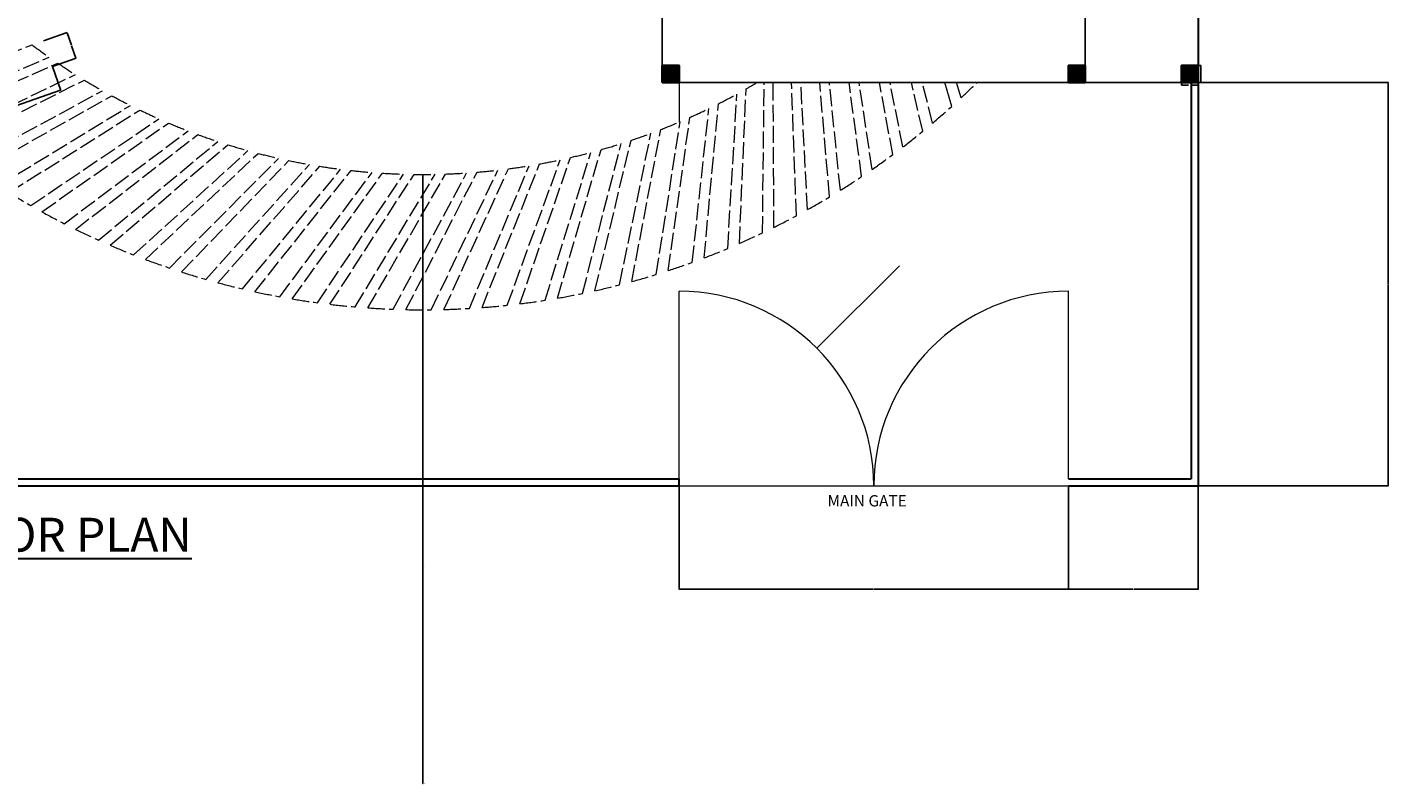
# Model space of a CAD drawing. Units: inches. Extents: x 2330 to 3943, y 1763 to 3461.
# Tile 12 of 40: x 2977 to 3943, y 1763 to 2300. Entities that reach past the tile are written whole.
import ezdxf

# ---------------------------------------------------------------- set-up
doc = ezdxf.new("R2010")
doc.units = ezdxf.units.IN
doc.linetypes.add('ACAD_ISO02W100', pattern=[15, 12, -3])
for name, color, linetype, lineweight in [('A-ANNO-DIMS', 2, 'Continuous', 18), ('A-ANNO-TEXT', 7, 'Continuous', 18), ('A-ANNO-TITL', 7, 'Continuous', 30), ('A-COLS', 7, 'Continuous', 35), ('A-FLOR', 7, 'Continuous', 25), ('C-PROP', 7, 'Continuous', 30), ('L-GATE', 4, 'Continuous', 18), ('L-PVMT', 9, 'Continuous', 18), ('L-PVMT-JOIN', 9, 'ACAD_ISO02W100', 13)]:
    doc.layers.add(name, color=color, linetype=linetype, lineweight=lineweight)
doc.styles.get("Standard").update_dxf_attribs({"font": 'arial.ttf'})
doc.dimstyles.get("Standard").update_dxf_attribs({"dimtxt": 0.18, "dimasz": 0.18, "dimexe": 0.18, "dimexo": 0.0625, "dimgap": 0.09, "dimtad": 0, "dimtih": 1, "dimtoh": 1, "dimdec": 4, "dimzin": 0, "dimdsep": 46, "dimtxsty": 'Standard', "dimcen": 0.09, "dimadec": 0, "dimazin": 0, "dimtfac": 1, "dimtdec": 4, "dimtofl": 0, "dimtmove": 0, "dimatfit": 3, "dimfxl": 1, "dimtolj": 1, "dimtzin": 0, "dimarcsym": 0})

# ---------------------------------------------------------------- blocks, each defined once
blk = doc.blocks.new('PAVER-RADIAL')
for p, q in [((0, 15.76), (109.7, 19.29)), ((8.7, 0), (118.23, 7.05))]:
    blk.add_line(p, q)
for radius, start, end in [(559.83, 207.9852, 209.8274), (463.83, 213.96986, 215.81207)]:
    blk.add_arc((494.37, 278.45), radius, start, end)
blk = doc.blocks.new('POST-PORCH-12IN')
h = blk.add_hatch(color=256)
h.dxf.hatch_style = 1
h.paths.add_polyline_path([(12, 12), (0, 12), (0, 0), (12, 0)])
blk.add_lwpolyline([(0, 0), (12, 0), (12, 12), (0, 12)], close=True)
blk = doc.blocks.new('*D25')
at = {"layer": 'A-ANNO-DIMS', "color": 0, "lineweight": -2, "transparency": 16777216}
for p, q in [((2994.99, 2271.94), (3000.9, 2255.1)), ((3000.67, 2255.21), (2945.58, 2235.87)), ((2883.43, 2232.78), (2889.34, 2215.93)), ((2889.45, 2216.16), (2944.54, 2235.5))]:
    blk.add_line(p, q, dxfattribs=at)
at = {"layer": 'A-ANNO-DIMS', "color": 0, "transparency": 16777216}
for points in [[(3000.66, 2255.23), (3000.68, 2255.18), (3000.84, 2255.27)], [(2889.44, 2216.19), (2889.46, 2216.14), (2889.28, 2216.1)]]:
    blk.add_solid(points, dxfattribs=at)
at = {"layer": 'Defpoints', "color": 0, "transparency": 16777216}
for p in [(2994.96, 2272), (3000.84, 2255.27), (2883.41, 2232.84)]:
    blk.add_point(p, dxfattribs=at)
at = {"layer": 'A-ANNO-DIMS', "color": 0, "transparency": 16777216, "insert": (2945.06, 2235.69), "char_height": 0.18, "attachment_point": 5}
blk.add_mtext('\\A1;PAVER 118 TYP.', dxfattribs=at)
blk = doc.blocks.new('*D26')
at = {"layer": 'A-ANNO-DIMS', "color": 0, "lineweight": -2, "transparency": 16777216}
for p, q in [((2988.64, 2290.22), (3005.48, 2296.13)), ((3005.37, 2295.9), (3008.44, 2287.15)), ((3011.64, 2278.04), (3008.57, 2286.79)), ((2995.02, 2272.02), (3011.87, 2277.93))]:
    blk.add_line(p, q, dxfattribs=at)
at = {"layer": 'A-ANNO-DIMS', "color": 0, "transparency": 16777216}
for points in [[(3005.4, 2295.91), (3005.34, 2295.89), (3005.31, 2296.07)], [(3011.67, 2278.05), (3011.61, 2278.03), (3011.7, 2277.87)]]:
    blk.add_solid(points, dxfattribs=at)
at = {"layer": 'Defpoints', "color": 0, "transparency": 16777216}
for p in [(2988.58, 2290.2), (3005.31, 2296.07), (2994.96, 2272)]:
    blk.add_point(p, dxfattribs=at)
at = {"layer": 'A-ANNO-DIMS', "color": 0, "transparency": 16777216, "insert": (3008.5, 2286.97), "char_height": 0.18, "attachment_point": 5}
blk.add_mtext('\\A1;19 TYP.', dxfattribs=at)
blk = doc.blocks.new('*D29')
at = {"layer": 'A-ANNO-DIMS', "color": 0, "lineweight": -2, "transparency": 16777216}
for p, q in [((3795.66, 2260.64), (3795.66, 2258.72)), ((3807.66, 2260.64), (3807.66, 2258.72)), ((3795.84, 2258.9), (3800.76, 2258.9)), ((3807.48, 2258.9), (3802.56, 2258.9))]:
    blk.add_line(p, q, dxfattribs=at)
at = {"layer": 'A-ANNO-DIMS', "color": 0, "transparency": 16777216}
for points in [[(3795.84, 2258.93), (3795.84, 2258.87), (3795.66, 2258.9)], [(3807.48, 2258.93), (3807.48, 2258.87), (3807.66, 2258.9)]]:
    blk.add_solid(points, dxfattribs=at)
at = {"layer": 'Defpoints', "color": 0, "transparency": 16777216}
for p in [(3795.66, 2260.7), (3807.66, 2260.7), (3807.66, 2258.9)]:
    blk.add_point(p, dxfattribs=at)
at = {"layer": 'A-ANNO-DIMS', "color": 0, "transparency": 16777216, "insert": (3801.66, 2258.9), "char_height": 0.18, "attachment_point": 5}
blk.add_mtext('\\A1;POST 12 TYP.', dxfattribs=at)
blk = doc.blocks.new('*D30')
at = {"layer": 'A-ANNO-DIMS', "color": 0, "lineweight": -2, "transparency": 16777216}
for p, q in [((3807.72, 2272.7), (3809.64, 2272.7)), ((3809.46, 2272.52), (3809.46, 2266.88)), ((3807.72, 2260.7), (3809.64, 2260.7)), ((3809.46, 2260.88), (3809.46, 2266.52))]:
    blk.add_line(p, q, dxfattribs=at)
at = {"layer": 'A-ANNO-DIMS', "color": 0, "transparency": 16777216}
for points in [[(3809.43, 2272.52), (3809.49, 2272.52), (3809.46, 2272.7)], [(3809.43, 2260.88), (3809.49, 2260.88), (3809.46, 2260.7)]]:
    blk.add_solid(points, dxfattribs=at)
at = {"layer": 'Defpoints', "color": 0, "transparency": 16777216}
for p in [(3807.66, 2272.7), (3809.46, 2272.7), (3807.66, 2260.7)]:
    blk.add_point(p, dxfattribs=at)
at = {"layer": 'A-ANNO-DIMS', "color": 0, "transparency": 16777216, "insert": (3809.46, 2266.7), "char_height": 0.18, "attachment_point": 5}
blk.add_mtext('\\A1;12 TYP.', dxfattribs=at)
blk = doc.blocks.new('*D65')
at = {"layer": 'A-ANNO-DIMS', "color": 0, "lineweight": -2, "transparency": 16777216}
for p, q in [((3439.52, 1974.59), (3439.52, 1901.2)), ((3715.52, 1974.59), (3715.52, 1901.2)), ((3439.7, 1901.38), (3577.23, 1901.38)), ((3715.34, 1901.38), (3577.81, 1901.38))]:
    blk.add_line(p, q, dxfattribs=at)
at = {"layer": 'A-ANNO-DIMS', "color": 0, "transparency": 16777216}
for points in [[(3439.7, 1901.41), (3439.7, 1901.35), (3439.52, 1901.38)], [(3715.34, 1901.41), (3715.34, 1901.35), (3715.52, 1901.38)]]:
    blk.add_solid(points, dxfattribs=at)
at = {"layer": 'Defpoints', "color": 0, "transparency": 16777216}
for p in [(3439.52, 1974.65), (3715.52, 1974.65), (3715.52, 1901.38)]:
    blk.add_point(p, dxfattribs=at)
at = {"layer": 'A-ANNO-DIMS', "color": 0, "transparency": 16777216, "insert": (3577.52, 1901.38), "char_height": 0.18, "attachment_point": 5}
blk.add_mtext('\\A1;276', dxfattribs=at)
blk = doc.blocks.new('*D66')
at = {"layer": 'A-ANNO-DIMS', "color": 0, "lineweight": -2, "transparency": 16777216}
for p, q in [((3715.52, 1974.59), (3715.52, 1901.2)), ((3807.66, 1974.59), (3807.66, 1901.2)), ((3715.7, 1901.38), (3761.19, 1901.38)), ((3807.48, 1901.38), (3761.98, 1901.38))]:
    blk.add_line(p, q, dxfattribs=at)
at = {"layer": 'A-ANNO-DIMS', "color": 0, "transparency": 16777216}
for points in [[(3715.7, 1901.41), (3715.7, 1901.35), (3715.52, 1901.38)], [(3807.48, 1901.41), (3807.48, 1901.35), (3807.66, 1901.38)]]:
    blk.add_solid(points, dxfattribs=at)
at = {"layer": 'Defpoints', "color": 0, "transparency": 16777216}
for p in [(3715.52, 1974.65), (3807.66, 1974.65), (3807.66, 1901.38)]:
    blk.add_point(p, dxfattribs=at)
at = {"layer": 'A-ANNO-DIMS', "color": 0, "transparency": 16777216, "insert": (3761.59, 1901.38), "char_height": 0.18, "attachment_point": 5}
blk.add_mtext('\\A1;92.14', dxfattribs=at)
blk = doc.blocks.new('*D68')
at = {"layer": 'A-ANNO-DIMS', "color": 0, "lineweight": -2, "transparency": 16777216}
for p, q in [((3807.72, 2260.7), (3942.54, 2260.7)), ((3942.36, 2260.52), (3942.36, 2117.86)), ((3942.36, 1974.83), (3942.36, 2117.5)), ((3807.72, 1974.65), (3942.54, 1974.65))]:
    blk.add_line(p, q, dxfattribs=at)
at = {"layer": 'A-ANNO-DIMS', "color": 0, "transparency": 16777216}
for points in [[(3942.33, 2260.52), (3942.39, 2260.52), (3942.36, 2260.7)], [(3942.33, 1974.83), (3942.39, 1974.83), (3942.36, 1974.65)]]:
    blk.add_solid(points, dxfattribs=at)
at = {"layer": 'Defpoints', "color": 0, "transparency": 16777216}
for p in [(3807.66, 2260.7), (3942.36, 2260.7), (3807.66, 1974.65)]:
    blk.add_point(p, dxfattribs=at)
at = {"layer": 'A-ANNO-DIMS', "color": 0, "transparency": 16777216, "insert": (3942.36, 2117.68), "char_height": 0.18, "attachment_point": 5}
blk.add_mtext('\\A1;286.05', dxfattribs=at)
blk = doc.blocks.new('*D103')
at = {"layer": 'A-ANNO-DIMS', "color": 0, "lineweight": -2, "transparency": 16777216}
for p, q in [((3257.55, 2659.32), (3257.73, 2659.32)), ((3257.64, 2659.23), (3257.64, 2659.41)), ((3257.66, 1763.59), (3257.65, 2099.31)), ((3257.84, 1763.59), (3257.66, 1763.59))]:
    blk.add_line(p, q, dxfattribs=at)
at = {"layer": 'A-ANNO-DIMS', "color": 0, "transparency": 16777216}
blk.add_solid([(3257.68, 2099.31), (3257.62, 2099.31), (3257.65, 2099.49)], dxfattribs=at)
at = {"layer": 'Defpoints', "color": 0, "transparency": 16777216}
for p in [(3257.64, 2659.32), (3257.65, 2099.49)]:
    blk.add_point(p, dxfattribs=at)
at = {"layer": 'A-ANNO-DIMS', "color": 0, "transparency": 16777216, "insert": (3258.58, 1763.59), "char_height": 0.18, "attachment_point": 5}
blk.add_mtext('\\A1;40X R559.8', dxfattribs=at)
blk = doc.blocks.new('*D104')
at = {"layer": 'A-ANNO-DIMS', "color": 0, "lineweight": -2, "transparency": 16777216}
for p, q in [((3257.55, 2659.32), (3257.73, 2659.32)), ((3257.64, 2659.23), (3257.64, 2659.41)), ((3257.66, 1917.19), (3257.65, 2195.31)), ((3257.84, 1917.19), (3257.66, 1917.19))]:
    blk.add_line(p, q, dxfattribs=at)
at = {"layer": 'A-ANNO-DIMS', "color": 0, "transparency": 16777216}
blk.add_solid([(3257.68, 2195.31), (3257.62, 2195.31), (3257.65, 2195.49)], dxfattribs=at)
at = {"layer": 'Defpoints', "color": 0, "transparency": 16777216}
for p in [(3257.64, 2659.32), (3257.65, 2195.49)]:
    blk.add_point(p, dxfattribs=at)
at = {"layer": 'A-ANNO-DIMS', "color": 0, "transparency": 16777216, "insert": (3258.58, 1917.19), "char_height": 0.18, "attachment_point": 5}
blk.add_mtext('\\A1;33X R463.8', dxfattribs=at)
blk = doc.blocks.new('*D105')
at = {"layer": 'A-ANNO-DIMS', "color": 0, "lineweight": -2, "transparency": 16777216}
for p, q in [((3595.65, 2130.78), (3537.22, 2072.36)), ((3595.83, 2130.78), (3595.65, 2130.78)), ((3439.43, 1974.65), (3439.61, 1974.65)), ((3439.52, 1974.56), (3439.52, 1974.74))]:
    blk.add_line(p, q, dxfattribs=at)
at = {"layer": 'A-ANNO-DIMS', "color": 0, "transparency": 16777216}
blk.add_solid([(3537.2, 2072.38), (3537.25, 2072.34), (3537.1, 2072.23)], dxfattribs=at)
at = {"layer": 'Defpoints', "color": 0, "transparency": 16777216}
for p in [(3537.1, 2072.23), (3439.52, 1974.65)]:
    blk.add_point(p, dxfattribs=at)
at = {"layer": 'A-ANNO-DIMS', "color": 0, "transparency": 16777216, "insert": (3596.4, 2130.78), "char_height": 0.18, "attachment_point": 5}
blk.add_mtext('\\A1;2X R138', dxfattribs=at)

msp = doc.modelspace()

# ---------------------------------------------------------------- linework, layer by layer
at = {"layer": 'A-FLOR'}
msp.add_line((3727.5159, 2260.7019), (3807.6605, 2260.7019), dxfattribs=at)
msp.add_lwpolyline([(3427.5159, 2260.7019), (3727.5159, 2260.7019), (3727.5159, 2560.7019), (3427.5159, 2560.7019)], close=True, dxfattribs=at)
at = {"layer": 'C-PROP'}
for p, q in [((3807.6605, 3210.6524), (3807.6605, 1974.6524)), ((3802.6605, 2260.7019), (3802.6605, 1979.6524)), ((2420.6605, 1979.6524), (3439.5159, 1979.6524)), ((3439.5159, 1974.6524), (3439.5159, 1979.6524)), ((3715.5159, 1979.6524), (3802.6605, 1979.6524)), ((2415.6605, 1974.6524), (3439.5159, 1974.6524)), ((3715.5159, 1974.6524), (3807.6605, 1974.6524))]:
    msp.add_line(p, q, dxfattribs=at)
at = {"layer": 'L-GATE'}
for p, q in [((3439.5159, 1979.6524), (3439.5159, 2112.6524)), ((3715.5159, 1979.6524), (3715.5159, 2112.6524)), ((3439.5159, 1974.6524), (3715.5159, 1974.6524))]:
    msp.add_line(p, q, dxfattribs=at)
for centre, start, end in [((3439.5159, 1974.6524), 360, 90), ((3715.5159, 1974.6524), 90, 180)]:
    msp.add_arc(centre, 138, start, end, dxfattribs=at)
at = {"layer": 'L-PVMT'}
for p, q in [((3439.5159, 2260.7019), (3439.5159, 2232.6357)), ((3632.7472, 2243.7426), (3627.9076, 2260.7019)), ((3639.3794, 2249.8263), (3636.086, 2260.7019))]:
    msp.add_line(p, q, dxfattribs=at)
at = {"layer": 'L-PVMT-JOIN'}
for p, q in [((3498.5655, 2153.9838), (3499.7818, 2260.7019)), ((3506.6579, 2157.9222), (3506.177, 2260.7019)), ((3522.6477, 2166.1865), (3519.165, 2260.7019)), ((3530.5409, 2170.5103), (3525.7646, 2260.7019)), ((3546.1137, 2179.5359), (3539.1929, 2260.7019)), ((3553.7892, 2184.2353), (3546.0291, 2260.7019)), ((3568.9087, 2194.0012), (3559.9652, 2260.7019)), ((3576.3488, 2199.0651), (3567.0733, 2260.7019)), ((3590.9799, 2209.5485), (3581.5913, 2260.7019)), ((3598.1672, 2214.9653), (3589.0104, 2260.7019)), ((3612.276, 2226.1419), (3604.1932, 2260.7019)), ((3619.1937, 2231.8988), (3611.9671, 2260.7019)), ((3482.1958, 2146.5), (3486.9742, 2256.1523))]:
    msp.add_line(p, q, dxfattribs=at)
for radius, start, end in [(463.831, 299.6324389, 300.7500144), (559.831, 312.9909402, 314.599268), (559.831, 310.2276312, 312.0698372), (559.831, 307.4643221, 309.3065282), (559.831, 304.7010131, 306.5432191), (559.831, 301.9377041, 303.7799101), (559.831, 299.1743951, 301.0166011), (559.831, 296.4110861, 298.2532921), (559.831, 293.647777, 295.489983)]:
    msp.add_arc((3257.6403, 2659.3212), radius, start, end, dxfattribs=at)

# ---------------------------------------------------------------- block references
at = {"layer": 'A-COLS'}
for p in [(3427.5159, 2260.7019), (3715.5159, 2260.7019), (3795.6605, 2260.7019)]:
    msp.add_blockref('POST-PORCH-12IN', p, dxfattribs=at)
at = {"layer": 'L-PVMT-JOIN'}
for p, rotation in [((2883.4084, 2232.8376), 19.34316315207948), ((2904.4044, 2215.2918), 22.10647217380505), ((2926.2218, 2198.7785), 24.86978119553056), ((2948.81, 2183.3363), 27.63309021683611), ((3472.8479, 2134.3226), 82.89927065654422), ((2972.1164, 2169.001), 30.39639923898183), ((3447.2874, 2124.5579), 80.13596163004335), ((2996.0868, 2155.806), 33.15970826070743), ((3421.2858, 2116.0368), 77.3726526083178), ((3020.6655, 2143.7819), 35.92301728243296), ((3045.7953, 2132.9568), 38.68632630415883), ((3368.2024, 2102.8018), 71.84603456486649), ((3394.9037, 2108.7791), 74.60934358659213), ((3071.4177, 2123.3558), 41.44963532588444), ((3097.4732, 2115.0012), 44.2129443476102), ((3341.244, 2098.1187), 69.08272554314082), ((3123.9012, 2107.9124), 46.97625336933581), ((3150.6402, 2102.106), 49.73956239106138), ((3177.6281, 2097.5954), 52.50287141278699), ((3204.802, 2094.3912), 55.26618043938523), ((3232.0988, 2092.5007), 58.02948945623847), ((3259.455, 2091.9285), 60.79279847796399), ((3286.807, 2092.6757), 63.55610749968956), ((3314.0911, 2094.7407), 66.3194165240299)]:
    msp.add_blockref('PAVER-RADIAL', p, dxfattribs=dict(at, rotation=rotation))

# ---------------------------------------------------------------- texts
at = {"layer": 'A-ANNO-TEXT', "insert": (3544.714, 1968.014), "char_height": 8, "attachment_point": 1}
msp.add_mtext_dynamic_manual_height_columns('MAIN GATE', width=541.30363, gutter_width=12.5, heights=[0], dxfattribs=at)
at = {"layer": 'A-ANNO-TITL', "insert": (2754.4138, 1951.9773), "char_height": 24, "attachment_point": 1}
msp.add_mtext_dynamic_manual_height_columns('{\\LGROUND FLOOR PLAN}', width=457.144969, gutter_width=12.5, heights=[0], dxfattribs=at)

# ---------------------------------------------------------------- dimensions: what is measured, and where the dimension line sits
at = {"layer": 'A-ANNO-DIMS'}
for center, mpoint, text, override, picture, middle in [((3257.6403, 2659.3212), (3257.65, 2099.4902), '40X <>', {"dimdec": 1, "dimlfac": 1, "dimrnd": 0, "dimzin": 0, "dimdsep": 46, "dimlunit": 2}, '*D103', (3258.5828, 1763.5916)), ((3257.6403, 2659.3212), (3257.65, 2195.4902), '33X <>', {"dimdec": 1, "dimlfac": 1, "dimrnd": 0, "dimzin": 0, "dimdsep": 46, "dimlunit": 2}, '*D104', (3258.5791, 1917.1916)), ((3439.5159, 1974.6524), (3537.0969, 2072.2329), '2X <>', {"dimdec": 0, "dimlfac": 1, "dimrnd": 0, "dimzin": 0, "dimdsep": 46, "dimlunit": 2}, '*D105', (3596.3956, 2130.7811))]:
    dim = msp.add_radius_dim(center=center, mpoint=mpoint, text=text, dimstyle='Standard', override=override, dxfattribs=at)
    dim.commit()
    dim.dimension.update_dxf_attribs({"geometry": picture, "text_midpoint": middle, "dimtype": 164})
for base, p1, p2, angle, text, picture, middle in [((3005.31, 2296.0694), (2994.9643, 2271.9988), (2988.5766, 2290.1953), 109.3431632, '<> TYP.', '*D26', (3008.5039, 2286.9711)), ((3000.8384, 2255.2654), (2883.4083, 2232.8381), (2994.9643, 2271.9988), 19.3431632, 'PAVER <> TYP.', '*D25', (2945.0604, 2235.685)), ((3809.4605, 2272.7019), (3807.6605, 2260.7019), (3807.6605, 2272.7019), 90, '<> TYP.', '*D30', (3809.4605, 2266.7019))]:
    dim = msp.add_linear_dim(base=base, p1=p1, p2=p2, angle=angle, text=text, dimstyle='Standard', override={"dimdec": 0, "dimlfac": 1, "dimrnd": 0, "dimzin": 0, "dimdsep": 46, "dimlunit": 2}, dxfattribs=at)
    dim.commit()
    dim.dimension.update_dxf_attribs({"geometry": picture, "text_midpoint": middle})
dim = msp.add_linear_dim(base=(3807.6605, 2258.9019), p1=(3795.6605, 2260.7019), p2=(3807.6605, 2260.7019), text='POST <> TYP.', dimstyle='Standard', override={"dimdec": 0, "dimlfac": 1, "dimrnd": 0, "dimzin": 0, "dimdsep": 46, "dimlunit": 2}, dxfattribs=at)
dim.commit()
dim.dimension.update_dxf_attribs({"geometry": '*D29', "text_midpoint": (3801.6605, 2258.9019)})
dim = msp.add_linear_dim(base=(3942.361, 2260.7019), p1=(3807.6605, 1974.6524), p2=(3807.6605, 2260.7019), angle=90, dimstyle='Standard', override={"dimdec": 2, "dimlfac": 1, "dimrnd": 0, "dimzin": 0, "dimdsep": 46, "dimlunit": 2}, dxfattribs=at)
dim.commit()
dim.dimension.update_dxf_attribs({"geometry": '*D68', "text_midpoint": (3942.361, 2117.6772)})
for base, p1, p2, override, picture, middle in [((3715.5159, 1901.3774), (3439.5159, 1974.6524), (3715.5159, 1974.6524), {"dimdec": 0, "dimlfac": 1, "dimrnd": 0, "dimzin": 0, "dimdsep": 46, "dimlunit": 2}, '*D65', (3577.5159, 1901.3774)), ((3807.6605, 1901.3774), (3715.5159, 1974.6524), (3807.6605, 1974.6524), {"dimdec": 2, "dimlfac": 1, "dimrnd": 0, "dimzin": 0, "dimdsep": 46, "dimlunit": 2}, '*D66', (3761.5882, 1901.3774))]:
    dim = msp.add_linear_dim(base=base, p1=p1, p2=p2, dimstyle='Standard', override=override, dxfattribs=at)
    dim.commit()
    dim.dimension.update_dxf_attribs({"geometry": picture, "text_midpoint": middle})

doc.saveas('drawing.dxf')
